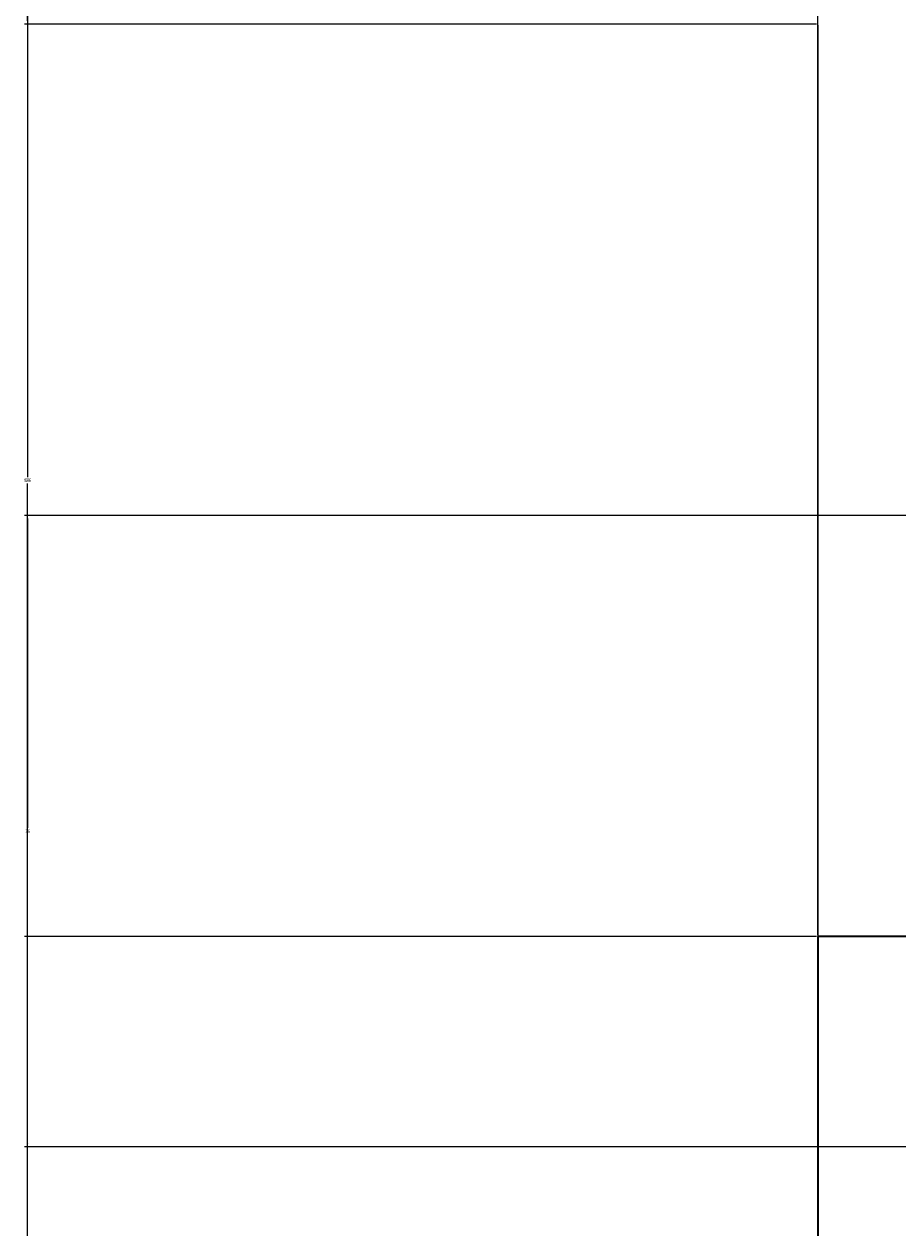
# Model space of a CAD drawing. Units: feet. Extents: x 105 to 1094, y -88 to 588.
# Tile 3 of 59: x 105 to 155, y 207 to 276. Entities that reach past the tile are written whole.
import ezdxf

# ---------------------------------------------------------------- set-up
doc = ezdxf.new("R2010")
doc.units = ezdxf.units.FT
doc.header["$MEASUREMENT"] = 0
doc.layers.add('A-ANNO-DIMS', color=2, linetype='Continuous', lineweight=18)
doc.layers.add('A-WALL', color=7, linetype='Continuous', lineweight=35)
doc.styles.get("Standard").update_dxf_attribs({"font": 'arial.ttf'})
doc.dimstyles.get("Standard").update_dxf_attribs({"dimtxt": 0.18, "dimasz": 0.18, "dimexe": 0.18, "dimexo": 0.0625, "dimgap": 0.09, "dimtad": 0, "dimtih": 1, "dimtoh": 1, "dimdec": 4, "dimzin": 0, "dimdsep": 46, "dimtxsty": 'Standard', "dimcen": 0.09, "dimadec": 0, "dimazin": 0, "dimtfac": 1, "dimtdec": 4, "dimtofl": 0, "dimtmove": 0, "dimatfit": 3, "dimfxl": 1, "dimtolj": 1, "dimtzin": 0, "dimarcsym": 0})

# ---------------------------------------------------------------- blocks, each defined once
blk = doc.blocks.new('*D20')
at = {"layer": 'A-ANNO-DIMS', "color": 0, "lineweight": -2, "transparency": 16777216}
for p, q in [((150.688, 276.019), (150.688, -88.149)), ((1048.688, 276.019), (1048.688, -88.149)), ((150.868, -87.969), (599.399, -87.969)), ((1048.508, -87.969), (599.977, -87.969))]:
    blk.add_line(p, q, dxfattribs=at)
at = {"layer": 'A-ANNO-DIMS', "color": 0, "transparency": 16777216}
for points in [[(150.868, -87.939), (150.868, -87.999), (150.688, -87.969)], [(1048.508, -87.939), (1048.508, -87.999), (1048.688, -87.969)]]:
    blk.add_solid(points, dxfattribs=at)
at = {"layer": 'Defpoints', "color": 0, "transparency": 16777216}
for p in [(150.688, 276.081), (1048.688, 276.081), (1048.688, -87.969)]:
    blk.add_point(p, dxfattribs=at)
at = {"layer": 'A-ANNO-DIMS', "color": 0, "transparency": 16777216, "insert": (599.688, -87.969), "char_height": 0.18, "attachment_point": 5}
blk.add_mtext('\\A1;898', dxfattribs=at)
blk = doc.blocks.new('*D21')
at = {"layer": 'A-ANNO-DIMS', "color": 0, "lineweight": -2, "transparency": 16777216}
for p, q in [((849.626, 543.081), (105.458, 543.081)), ((105.638, 542.901), (105.638, 250.263)), ((105.638, -42.739), (105.638, 249.899)), ((849.626, -42.919), (105.458, -42.919))]:
    blk.add_line(p, q, dxfattribs=at)
at = {"layer": 'A-ANNO-DIMS', "color": 0, "transparency": 16777216}
for points in [[(105.608, 542.901), (105.668, 542.901), (105.638, 543.081)], [(105.608, -42.739), (105.668, -42.739), (105.638, -42.919)]]:
    blk.add_solid(points, dxfattribs=at)
at = {"layer": 'Defpoints', "color": 0, "transparency": 16777216}
for p in [(105.638, 543.081), (849.688, 543.081), (849.688, -42.919)]:
    blk.add_point(p, dxfattribs=at)
at = {"layer": 'A-ANNO-DIMS', "color": 0, "transparency": 16777216, "insert": (105.638, 250.081), "char_height": 0.18, "attachment_point": 5}
blk.add_mtext('\\A1;586', dxfattribs=at)
blk = doc.blocks.new('*D28')
at = {"layer": 'A-ANNO-DIMS', "color": 0, "lineweight": -2, "transparency": 16777216}
for p, q in [((150.626, 424.081), (105.458, 424.081)), ((105.638, 423.901), (105.638, 350.263)), ((105.638, 276.261), (105.638, 349.899)), ((150.626, 276.081), (105.458, 276.081))]:
    blk.add_line(p, q, dxfattribs=at)
at = {"layer": 'A-ANNO-DIMS', "color": 0, "transparency": 16777216}
for points in [[(105.608, 423.901), (105.668, 423.901), (105.638, 424.081)], [(105.608, 276.261), (105.668, 276.261), (105.638, 276.081)]]:
    blk.add_solid(points, dxfattribs=at)
at = {"layer": 'Defpoints', "color": 0, "transparency": 16777216}
for p in [(105.638, 424.081), (150.688, 424.081), (150.688, 276.081)]:
    blk.add_point(p, dxfattribs=at)
at = {"layer": 'A-ANNO-DIMS', "color": 0, "transparency": 16777216, "insert": (105.638, 350.081), "char_height": 0.18, "attachment_point": 5}
blk.add_mtext('\\A1;148', dxfattribs=at)
blk = doc.blocks.new('*D29')
at = {"layer": 'A-ANNO-DIMS', "color": 0, "lineweight": -2, "transparency": 16777216}
for p, q in [((150.626, 276.081), (105.458, 276.081)), ((105.638, 275.901), (105.638, 250.263)), ((105.638, 224.261), (105.638, 249.899)), ((150.626, 224.081), (105.458, 224.081))]:
    blk.add_line(p, q, dxfattribs=at)
at = {"layer": 'A-ANNO-DIMS', "color": 0, "transparency": 16777216}
for points in [[(105.608, 275.901), (105.668, 275.901), (105.638, 276.081)], [(105.608, 224.261), (105.668, 224.261), (105.638, 224.081)]]:
    blk.add_solid(points, dxfattribs=at)
at = {"layer": 'Defpoints', "color": 0, "transparency": 16777216}
for p in [(105.638, 276.081), (150.688, 276.081), (150.688, 224.081)]:
    blk.add_point(p, dxfattribs=at)
at = {"layer": 'A-ANNO-DIMS', "color": 0, "transparency": 16777216, "insert": (105.638, 250.081), "char_height": 0.18, "attachment_point": 5}
blk.add_mtext('\\A1;52', dxfattribs=at)
blk = doc.blocks.new('*D36')
at = {"layer": 'A-ANNO-DIMS', "color": 0, "lineweight": -2, "transparency": 16777216}
for p, q in [((547.235, 248.081), (105.458, 248.081)), ((105.638, 247.901), (105.638, 230.263)), ((105.638, 212.261), (105.638, 229.899)), ((546.626, 212.081), (105.458, 212.081))]:
    blk.add_line(p, q, dxfattribs=at)
at = {"layer": 'A-ANNO-DIMS', "color": 0, "transparency": 16777216}
for points in [[(105.608, 247.901), (105.668, 247.901), (105.638, 248.081)], [(105.608, 212.261), (105.668, 212.261), (105.638, 212.081)]]:
    blk.add_solid(points, dxfattribs=at)
at = {"layer": 'Defpoints', "color": 0, "transparency": 16777216}
for p in [(105.638, 248.081), (547.298, 248.081), (546.688, 212.081)]:
    blk.add_point(p, dxfattribs=at)
at = {"layer": 'A-ANNO-DIMS', "color": 0, "transparency": 16777216, "insert": (105.638, 230.081), "char_height": 0.18, "attachment_point": 5}
blk.add_mtext('\\A1;36', dxfattribs=at)
blk = doc.blocks.new('*D38')
at = {"layer": 'A-ANNO-DIMS', "color": 0, "lineweight": -2, "transparency": 16777216}
for p, q in [((150.688, 224.144), (150.688, 588.311)), ((150.868, 588.131), (222.408, 588.131)), ((294.508, 588.131), (222.968, 588.131)), ((294.688, 224.144), (294.688, 588.311))]:
    blk.add_line(p, q, dxfattribs=at)
at = {"layer": 'A-ANNO-DIMS', "color": 0, "transparency": 16777216}
for points in [[(150.868, 588.161), (150.868, 588.101), (150.688, 588.131)], [(294.508, 588.161), (294.508, 588.101), (294.688, 588.131)]]:
    blk.add_solid(points, dxfattribs=at)
at = {"layer": 'Defpoints', "color": 0, "transparency": 16777216}
for p in [(294.688, 588.131), (150.688, 224.081), (294.688, 224.081)]:
    blk.add_point(p, dxfattribs=at)
at = {"layer": 'A-ANNO-DIMS', "color": 0, "transparency": 16777216, "insert": (222.688, 588.131), "char_height": 0.18, "attachment_point": 5}
blk.add_mtext('\\A1;144', dxfattribs=at)

msp = doc.modelspace()

# ---------------------------------------------------------------- linework, layer by layer
at = {"layer": 'A-WALL'}
for p, q in [((294.6883, 224.0812), (150.6883, 224.0812)), ((150.6883, 224.0812), (150.6883, 106.0812))]:
    msp.add_line(p, q, dxfattribs=at)

# ---------------------------------------------------------------- dimensions: what is measured, and where the dimension line sits
at = {"layer": 'A-ANNO-DIMS'}
for base, p1, p2, picture, middle in [((294.6883, 588.1312), (150.6883, 224.0812), (294.6883, 224.0812), '*D38', (222.6883, 588.1312)), ((1048.6883, -87.9688), (150.6883, 276.0812), (1048.6883, 276.0812), '*D20', (599.6883, -87.9688))]:
    dim = msp.add_linear_dim(base=base, p1=p1, p2=p2, dimstyle='Standard', override={"dimdec": 0, "dimlfac": 1, "dimrnd": 0, "dimzin": 0, "dimdsep": 46, "dimlunit": 2}, dxfattribs=at)
    dim.commit()
    dim.dimension.update_dxf_attribs({"geometry": picture, "text_midpoint": middle})
for base, p1, p2, picture, middle in [((105.6383, 543.0812), (849.6883, -42.9188), (849.6883, 543.0812), '*D21', (105.6383, 250.0812)), ((105.6383, 424.0812), (150.6883, 276.0812), (150.6883, 424.0812), '*D28', (105.6383, 350.0812)), ((105.6383, 276.0812), (150.6883, 224.0812), (150.6883, 276.0812), '*D29', (105.6383, 250.0812)), ((105.6383, 248.0812), (546.6883, 212.0812), (547.2975, 248.0812), '*D36', (105.6383, 230.0812))]:
    dim = msp.add_linear_dim(base=base, p1=p1, p2=p2, angle=90, dimstyle='Standard', override={"dimdec": 0, "dimlfac": 1, "dimrnd": 0, "dimzin": 0, "dimdsep": 46, "dimlunit": 2}, dxfattribs=at)
    dim.commit()
    dim.dimension.update_dxf_attribs({"geometry": picture, "text_midpoint": middle})

doc.saveas('drawing.dxf')
